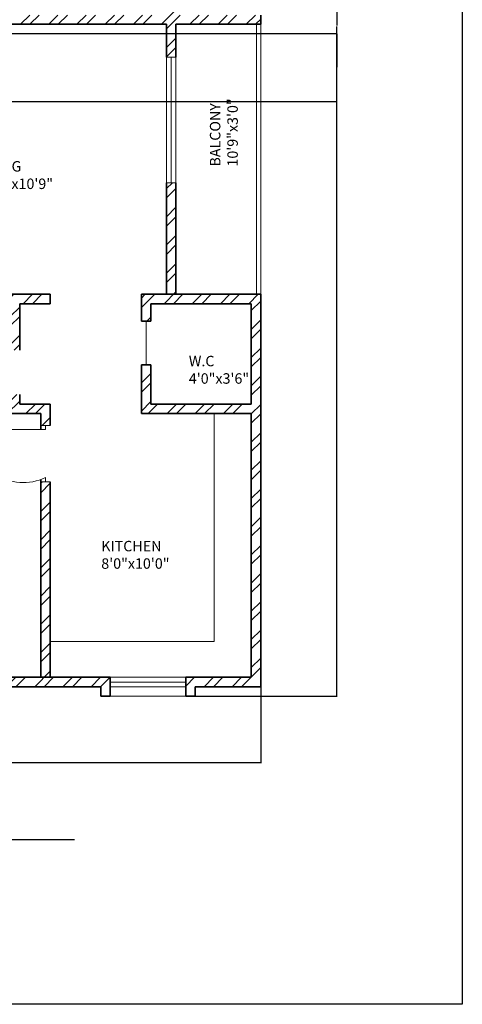
# Model space of a CAD drawing. Units: inches. Extents: x 1570 to 2186, y 1575 to 2421.
# Tile 5 of 10: x 1975 to 2186, y 1575 to 2045. Entities that reach past the tile are written whole.
import ezdxf

# ---------------------------------------------------------------- set-up
doc = ezdxf.new("R2010")
doc.units = ezdxf.units.IN
for name, color, linetype, lineweight in [('A-ANNO-DIMS', 2, 'Continuous', 18), ('A-ANNO-TTLB', 7, 'Continuous', 25), ('A-AREA-IDEN', 7, 'Continuous', 18), ('A-DOOR', 201, 'Continuous', 18), ('A-FLOR-CASE', 7, 'Continuous', 18), ('A-FLOR-HRAL', 201, 'Continuous', 18), ('A-GLAZ', 150, 'Continuous', 18), ('A-WALL', 7, 'Continuous', 35), ('A-WALL-PATT', 252, 'Continuous', 13)]:
    doc.layers.add(name, color=color, linetype=linetype, lineweight=lineweight)
doc.styles.get("Standard").update_dxf_attribs({"font": 'arial.ttf'})
doc.dimstyles.get("Standard").update_dxf_attribs({"dimtxt": 0.18, "dimasz": 0.18, "dimexe": 0.18, "dimexo": 0.0625, "dimgap": 0.09, "dimtad": 0, "dimtih": 1, "dimtoh": 1, "dimdec": 4, "dimzin": 0, "dimdsep": 46, "dimtxsty": 'Standard', "dimcen": 0.09, "dimadec": 0, "dimazin": 0, "dimtfac": 1, "dimtdec": 4, "dimtofl": 0, "dimtmove": 0, "dimatfit": 3, "dimfxl": 1, "dimtolj": 1, "dimtzin": 0, "dimarcsym": 0})

# ---------------------------------------------------------------- blocks, each defined once
blk = doc.blocks.new('WIN-60IN')
for p, q in [((0, 60), (4.5, 60)), ((0, 0), (0, 60)), ((4.5, 60), (2.25, 60)), ((2.25, 60), (2.25, 0)), ((4.5, 60), (4.5, 0)), ((2.25, 0), (0, 0)), ((0, 0), (4.5, 0))]:
    blk.add_line(p, q)
blk = doc.blocks.new('*D31')
at = {"layer": 'A-ANNO-DIMS', "color": 0, "lineweight": -2, "transparency": 16777216}
for p, q in [((1639.59, 1726.19), (1639.59, 1689.77)), ((2090.09, 1726.19), (2090.09, 1689.77)), ((1639.77, 1689.95), (1864.44, 1689.95)), ((2089.91, 1689.95), (1865.24, 1689.95))]:
    blk.add_line(p, q, dxfattribs=at)
at = {"layer": 'A-ANNO-DIMS', "color": 0, "transparency": 16777216}
for points in [[(1639.77, 1689.98), (1639.77, 1689.92), (1639.59, 1689.95)], [(2089.91, 1689.98), (2089.91, 1689.92), (2090.09, 1689.95)]]:
    blk.add_solid(points, dxfattribs=at)
at = {"layer": 'Defpoints', "color": 0, "transparency": 16777216}
for p in [(1639.59, 1726.25), (2090.09, 1726.25), (1639.59, 1689.95)]:
    blk.add_point(p, dxfattribs=at)
at = {"layer": 'A-ANNO-DIMS', "color": 0, "transparency": 16777216, "insert": (1864.84, 1689.95), "char_height": 0.18, "attachment_point": 5}
blk.add_mtext('\\A1;450.5', dxfattribs=at)
blk = doc.blocks.new('*D32')
at = {"layer": 'A-ANNO-DIMS', "color": 0, "lineweight": -2, "transparency": 16777216}
for p, q in [((2053.61, 2362.15), (2126.57, 2362.15)), ((2126.39, 2361.97), (2126.39, 2042.13)), ((2126.39, 1721.93), (2126.39, 2041.77)), ((2058.81, 1721.75), (2126.57, 1721.75))]:
    blk.add_line(p, q, dxfattribs=at)
at = {"layer": 'A-ANNO-DIMS', "color": 0, "transparency": 16777216}
for points in [[(2126.36, 2361.97), (2126.42, 2361.97), (2126.39, 2362.15)], [(2126.36, 1721.93), (2126.42, 1721.93), (2126.39, 1721.75)]]:
    blk.add_solid(points, dxfattribs=at)
at = {"layer": 'Defpoints', "color": 0, "transparency": 16777216}
for p in [(2053.54, 2362.15), (2126.39, 2362.15), (2058.75, 1721.75)]:
    blk.add_point(p, dxfattribs=at)
at = {"layer": 'A-ANNO-DIMS', "color": 0, "transparency": 16777216, "insert": (2126.39, 2041.95), "char_height": 0.18, "attachment_point": 5}
blk.add_mtext('\\A1;640.4', dxfattribs=at)
blk = doc.blocks.new('*D41')
at = {"layer": 'A-ANNO-DIMS', "color": 0, "lineweight": -2, "transparency": 16777216}
for p, q in [((1816.15, 2038.3), (2126.57, 2038.3)), ((2126.39, 2038.12), (2126.39, 2022.3)), ((2126.39, 2006.11), (2126.39, 2021.93)), ((1816.15, 2005.93), (2126.57, 2005.93))]:
    blk.add_line(p, q, dxfattribs=at)
at = {"layer": 'A-ANNO-DIMS', "color": 0, "transparency": 16777216}
for points in [[(2126.36, 2038.12), (2126.42, 2038.12), (2126.39, 2038.3)], [(2126.36, 2006.11), (2126.42, 2006.11), (2126.39, 2005.93)]]:
    blk.add_solid(points, dxfattribs=at)
at = {"layer": 'Defpoints', "color": 0, "transparency": 16777216}
for p in [(1816.09, 2038.3), (2126.39, 2038.3), (1816.09, 2005.93)]:
    blk.add_point(p, dxfattribs=at)
at = {"layer": 'A-ANNO-DIMS', "color": 0, "transparency": 16777216, "insert": (2126.39, 2022.12), "char_height": 0.18, "attachment_point": 5}
blk.add_mtext('\\A1;32.365', dxfattribs=at)

msp = doc.modelspace()

# ---------------------------------------------------------------- hatches: boundary and pattern name
at = {"layer": 'A-WALL-PATT'}
h = msp.add_hatch(dxfattribs=at)
h.set_pattern_fill('ANSI32', color=256)
h.paths.add_polyline_path([(1762.0975, 2362.1492), (1757.5975, 2362.1492), (1757.5975, 2357.6492), (1709.1163, 2357.6492), (1709.1163, 2362.1492), (1704.6163, 2362.1492), (1704.6163, 2353.1492), (1740.0886, 2353.1492), (1740.0886, 2261.8115), (1744.5886, 2261.8115), (1744.5886, 2353.1492), (1762.0975, 2353.1492)])
h.paths.add_polyline_path([(1890.2592, 2362.1492), (1885.7592, 2362.1492), (1826.5975, 2362.1492), (1822.0975, 2362.1492), (1822.0975, 2353.1492), (1862.5886, 2353.1492), (1862.5886, 2227.1492), (1744.5886, 2227.1492), (1744.5886, 2229.5389), (1742.3386, 2229.5389), (1740.0886, 2229.5389), (1740.0886, 2222.6492), (1744.5886, 2222.6492), (1756.186, 2222.6492), (1756.186, 2216.3571), (1760.686, 2216.3571), (1760.686, 2222.6492), (1832.686, 2222.6492), (1832.686, 2212.5994), (1837.186, 2212.5994), (1837.186, 2222.6492), (1893.186, 2222.6492), (1893.186, 2212.5994), (1897.686, 2212.5994), (1897.686, 2222.6492), (1989.5886, 2222.6492), (1989.5886, 2227.1492), (1989.5886, 2232.6585), (1987.3386, 2232.6585), (1985.0886, 2232.6585), (1985.0886, 2227.1492), (1867.0886, 2227.1492), (1867.0886, 2353.1492), (1890.2592, 2353.1492)])
h.paths.add_polyline_path([(1644.0886, 2353.1492), (1668.6163, 2353.1492), (1668.6163, 2362.1492), (1664.1163, 2362.1492), (1664.1163, 2358.9932), (1664.1163, 2357.6492), (1639.5886, 2357.6492), (1639.5886, 2213.8746), (1644.0886, 2213.8746), (1644.0886, 2222.6492), (1692.0886, 2222.6492), (1692.0886, 2215.9343), (1696.5886, 2215.9343), (1696.5886, 2222.6492), (1696.5886, 2227.1492), (1644.0886, 2227.1492)])
h.paths.add_polyline_path([(2013.0435, 2362.1492), (2008.5435, 2362.1492), (2008.5435, 2357.6492), (1954.7592, 2357.6492), (1954.7592, 2362.1492), (1950.2592, 2362.1492), (1950.2592, 2353.1492), (1985.0886, 2353.1492), (1985.0886, 2260.8534), (1989.5886, 2260.8534), (1989.5886, 2353.1492), (2013.0435, 2353.1492)])
h.paths.add_polyline_path([(2090.0886, 2357.6492), (2053.5435, 2357.6492), (2053.5435, 2362.1492), (2049.0435, 2362.1492), (2049.0435, 2353.1492), (2085.5886, 2353.1492), (2085.5886, 2227.1492), (2033.0886, 2227.1492), (2033.0886, 2222.6492), (2033.0886, 2214.4464), (2037.5886, 2214.4464), (2037.5886, 2222.6492), (2085.5886, 2222.6492), (2085.5886, 2212.4409), (2090.0886, 2212.4409)])
h.paths.add_polyline_path([(2090.0886, 2188.4409), (2087.8386, 2188.4409), (2085.5886, 2188.4409), (2085.5886, 2180.6492), (2037.5886, 2180.6492), (2037.5886, 2196.7956), (2033.0886, 2196.7956), (2033.0886, 2176.1492), (2037.5886, 2176.1492), (2045.0886, 2176.1492), (2045.0886, 2169.8988), (2049.5886, 2169.8988), (2049.5886, 2176.1492), (2085.5886, 2176.1492), (2085.5886, 2167.785), (2090.0886, 2167.785)])
h.paths.add_polyline_path([(2049.5886, 2147.4502), (2047.3386, 2147.4502), (2045.0886, 2147.4502), (2045.0886, 2124.4703), (2049.5886, 2124.4703)])
h.paths.add_polyline_path([(2090.0886, 2047.1492), (2049.5886, 2047.1492), (2049.5886, 2064.4703), (2045.0886, 2064.4703), (2045.0886, 2047.1492), (1918.0886, 2047.1492), (1918.0886, 2051.2061), (1913.5886, 2051.2061), (1913.5886, 2047.1492), (1913.5886, 2036.6872), (1918.0886, 2036.6872), (1918.0886, 2042.7492), (2045.0886, 2042.7492), (2045.0886, 2027.0686), (2049.5886, 2027.0686), (2049.5886, 2042.7492), (2090.0886, 2042.7492)])
h.paths.add_polyline_path([(1918.0886, 2005.9338), (1915.8386, 2005.9338), (1913.5886, 2005.9338), (1913.5886, 1913.7492), (1918.0886, 1913.7492)])
h.paths.add_polyline_path([(2090.0886, 1913.7492), (2049.5886, 1913.7492), (2045.0886, 1913.7492), (2033.0886, 1913.7492), (2033.0886, 1909.2492), (2033.0886, 1900.9803), (2037.5886, 1900.9803), (2037.5886, 1909.2492), (2085.5886, 1909.2492), (2085.5886, 1861.2492), (2037.5886, 1861.2492), (2037.5886, 1880.0859), (2033.0886, 1880.0859), (2033.0886, 1856.7492), (2085.5886, 1856.7492), (2085.5886, 1730.7492), (2054.2483, 1730.7492), (2054.2483, 1721.7492), (2058.7483, 1721.7492), (2058.7483, 1726.2492), (2090.0886, 1726.2492)])
h.paths.add_polyline_path([(2049.5886, 1967.0686), (2045.0886, 1967.0686), (2045.0886, 1913.7492), (2049.5886, 1913.7492)])
h.paths.add_polyline_path([(1989.5886, 1824.1695), (1987.3386, 1824.1695), (1985.0886, 1824.1695), (1985.0886, 1730.7492), (1989.5886, 1730.7492)])
h.paths.add_polyline_path([(1989.5886, 1861.2492), (1974.9963, 1861.2492), (1974.9963, 1865.9306), (1972.7463, 1865.9306), (1970.4963, 1865.9306), (1970.4963, 1861.2492), (1898.4963, 1861.2492), (1898.4963, 1874.2999), (1893.9963, 1874.2999), (1893.9963, 1861.2492), (1890.5886, 1861.2492), (1837.9963, 1861.2492), (1837.9963, 1874.3159), (1833.4963, 1874.3159), (1833.4963, 1861.2492), (1761.4963, 1861.2492), (1761.4963, 1865.0209), (1759.2463, 1865.0209), (1756.9963, 1865.0209), (1756.9963, 1861.2492), (1740.0886, 1861.2492), (1740.0886, 1856.7492), (1740.0886, 1850.7206), (1744.5886, 1850.7206), (1744.5886, 1856.7492), (1985.0886, 1856.7492), (1985.0886, 1851.0804), (1989.5886, 1851.0804), (1989.5886, 1856.7492)])
h.paths.add_polyline_path([(1989.5886, 1913.7492), (1740.0886, 1913.7492), (1740.0886, 1909.2492), (1756.9963, 1909.2492), (1756.9963, 1890.279), (1761.4963, 1890.279), (1761.4963, 1909.2492), (1833.4963, 1909.2492), (1833.4963, 1898.3159), (1837.9963, 1898.3159), (1837.9963, 1909.2492), (1890.5886, 1909.2492), (1893.9963, 1909.2492), (1893.9963, 1898.2999), (1898.4963, 1898.2999), (1898.4963, 1909.2492), (1970.4963, 1909.2492), (1970.4963, 1886.9887), (1974.9963, 1886.9887), (1974.9963, 1909.2492), (1989.5886, 1909.2492)])
h.paths.add_polyline_path([(1893.7344, 1730.7492), (1867.0886, 1730.7492), (1867.0886, 1856.7492), (1862.5886, 1856.7492), (1862.5886, 1730.7492), (1824.0492, 1730.7492), (1824.0492, 1721.7492), (1893.7344, 1721.7492)])
h.paths.add_polyline_path([(2018.2483, 1730.7492), (1953.7344, 1730.7492), (1953.7344, 1721.7492), (1958.2344, 1721.7492), (1958.2344, 1726.2492), (2013.7483, 1726.2492), (2013.7483, 1721.7492), (2018.2483, 1721.7492)])
h.paths.add_polyline_path([(1768.5492, 1730.7492), (1764.0492, 1730.7492), (1744.5886, 1730.7492), (1744.5886, 1819.4364), (1742.3386, 1819.4364), (1740.0886, 1819.4364), (1740.0886, 1730.7492), (1697.3801, 1730.7492), (1697.3801, 1721.7492), (1701.8801, 1721.7492), (1701.8801, 1726.2492), (1764.0492, 1726.2492), (1764.0492, 1721.7492), (1768.5492, 1721.7492)])
h.paths.add_polyline_path([(1644.0886, 1856.7492), (1639.5886, 1856.7492), (1639.5886, 1726.2492), (1657.0315, 1726.2492), (1657.0315, 1721.7492), (1661.3801, 1721.7492), (1661.3801, 1730.7492), (1644.0886, 1730.7492)])
h.paths.add_polyline_path([(1696.5886, 1876.1809), (1692.0886, 1876.1809), (1692.0886, 1861.2492), (1684.5886, 1861.2492), (1644.0886, 1861.2492), (1644.0886, 1909.2492), (1692.0886, 1909.2492), (1692.0886, 1900.3394), (1696.5886, 1900.3394), (1696.5886, 1913.7492), (1684.5886, 1913.7492), (1684.5886, 1920.2115), (1682.3386, 1920.2115), (1680.0886, 1920.2115), (1680.0886, 1913.7492), (1639.5886, 1913.7492), (1639.5886, 1856.7492), (1684.5886, 1856.7492), (1692.0886, 1856.7492), (1696.5886, 1856.7492)])
h.paths.add_polyline_path([(1684.5886, 2042.7492), (1811.5886, 2042.7492), (1811.5886, 2038.2991), (1816.0886, 2038.2991), (1816.0886, 2042.7492), (1816.0886, 2052.5708), (1813.8386, 2052.5708), (1811.5886, 2052.5708), (1811.5886, 2047.1492), (1684.5886, 2047.1492), (1684.5886, 2064.4703), (1680.0886, 2064.4703), (1680.0886, 2047.1492), (1639.5886, 2047.1492), (1639.5886, 2042.7492), (1680.0886, 2042.7492), (1680.0886, 2024.0762), (1684.5886, 2024.0762)])
h.paths.add_polyline_path([(1684.5886, 1964.0762), (1680.0886, 1964.0762), (1680.0886, 1944.6145), (1684.5886, 1944.6145)])
h.paths.add_polyline_path([(1816.0886, 1973.7492), (1876.0886, 1973.7492), (1876.0886, 1959.17), (1880.5886, 1959.17), (1880.5886, 1973.7492), (1880.5886, 1978.2492), (1816.0886, 1978.2492), (1816.0886, 2005.9338), (1813.8386, 2005.9338), (1811.5886, 2005.9338), (1811.5886, 1913.7492), (1816.0886, 1913.7492)])
h.paths.add_polyline_path([(1837.186, 2180.6492), (1837.186, 2188.5994), (1834.936, 2188.5994), (1832.686, 2188.5994), (1832.686, 2180.6492), (1760.686, 2180.6492), (1760.686, 2197.4807), (1756.186, 2197.4807), (1756.186, 2180.6492), (1744.5886, 2180.6492), (1740.0886, 2180.6492), (1740.0886, 2176.1492), (1837.186, 2176.1492)])
h.paths.add_polyline_path([(1974.186, 2196.8744), (1971.936, 2196.8744), (1969.686, 2196.8744), (1969.686, 2180.6492), (1897.686, 2180.6492), (1897.686, 2188.5994), (1895.436, 2188.5994), (1893.186, 2188.5994), (1893.186, 2180.6492), (1893.186, 2176.1492), (1974.186, 2176.1492)])
h.paths.add_polyline_path([(1918.0886, 2176.1492), (1913.5886, 2176.1492), (1913.5886, 2081.3709), (1918.0886, 2081.3709)])
h.paths.add_polyline_path([(1816.0886, 2176.1492), (1811.5886, 2176.1492), (1811.5886, 2081.3709), (1816.0886, 2081.3709)])
h.paths.add_polyline_path([(1684.5886, 2150.4939), (1682.3386, 2150.4939), (1680.0886, 2150.4939), (1680.0886, 2124.4703), (1684.5886, 2124.4703)])
h.paths.add_polyline_path([(1696.5886, 2180.6492), (1696.5886, 2197.4701), (1692.0886, 2197.4701), (1692.0886, 2180.6492), (1644.0886, 2180.6492), (1644.0886, 2189.8746), (1641.8386, 2189.8746), (1639.5886, 2189.8746), (1639.5886, 2169.814), (1644.0886, 2169.814), (1644.0886, 2176.1492), (1680.0886, 2176.1492), (1680.0886, 2171.7002), (1684.5886, 2171.7002), (1684.5886, 2176.1492), (1696.5886, 2176.1492)])

# ---------------------------------------------------------------- linework, layer by layer
at = {"layer": 'A-ANNO-TTLB'}
msp.add_line((1731.492, 1653.2104), (2001.1233, 1653.2104), dxfattribs=at)
msp.add_lwpolyline([(1569.8198, 2421.0436), (2186.3437, 2421.0436), (2186.3437, 1574.5084), (1569.8198, 1574.5084)], close=True, dxfattribs=at)
at = {"layer": 'A-DOOR'}
for p, q in [((2035.3386, 1880.0859), (2035.3386, 1900.9803)), ((1987.3386, 1849.0804), (1951.3386, 1849.0804)), ((1985.0886, 1851.0804), (1989.5886, 1851.0804)), ((1989.5886, 1851.0804), (1987.3386, 1851.0804)), ((1987.3386, 1851.0804), (1987.3386, 1849.0804)), ((1987.3386, 1824.1695), (1987.3386, 1826.1695)), ((1985.0886, 1824.1695), (1989.5886, 1824.1695)), ((1989.5886, 1824.1695), (1987.3386, 1824.1695))]:
    msp.add_line(p, q, dxfattribs=at)
msp.add_arc((1976.629, 1849.0804), 25.2904, 180, 295.053575, dxfattribs=at)
at = {"layer": 'A-FLOR-CASE'}
for p, q in [((2067.9297, 1747.7768), (2067.9297, 1856.7492)), ((1989.5886, 1747.7768), (2067.9297, 1747.7768))]:
    msp.add_line(p, q, dxfattribs=at)
at = {"layer": 'A-FLOR-HRAL'}
for p, q in [((2087.998, 1913.7492), (2087.998, 2042.7492)), ((2090.0886, 1913.7492), (2090.0886, 2042.7492))]:
    msp.add_line(p, q, dxfattribs=at)
at = {"layer": 'A-GLAZ'}
for p, q in [((2018.2483, 1730.7492), (2054.2483, 1730.7492)), ((2018.2483, 1728.4649), (2054.2483, 1728.4649)), ((2054.2483, 1726.2492), (2018.2483, 1726.2492)), ((2018.2483, 1721.7492), (2054.2483, 1721.7492))]:
    msp.add_line(p, q, dxfattribs=at)
at = {"layer": 'A-WALL'}
for p, q in [((2090.0886, 2047.1492), (2090.0886, 2042.7492)), ((2045.0886, 2042.7492), (1918.0886, 2042.7492)), ((2045.0886, 2042.7492), (2037.5886, 2042.7492)), ((2045.0886, 2042.7492), (2045.0886, 2027.0686)), ((2090.0886, 2042.7492), (2049.5886, 2042.7492)), ((2049.5886, 2042.7492), (2049.5886, 2027.0686)), ((2045.0886, 1967.0686), (2045.0886, 1913.7492)), ((2049.5886, 1967.0686), (2049.5886, 1913.7492)), ((1989.5886, 1913.7492), (1740.0886, 1913.7492)), ((1989.5886, 1909.2492), (1989.5886, 1913.7492)), ((2085.5886, 1913.7492), (2033.0886, 1913.7492)), ((2033.0886, 1909.2492), (2033.0886, 1913.7492)), ((2049.5886, 1913.7492), (2045.0886, 1913.7492)), ((2090.0886, 1913.7492), (2049.5886, 1913.7492)), ((2090.0886, 1913.7492), (2090.0886, 1726.2492)), ((1989.5886, 1909.2492), (1974.9963, 1909.2492)), ((1974.9963, 1886.9887), (1974.9963, 1909.2492)), ((2033.0886, 1900.9803), (2033.0886, 1909.2492)), ((2085.5886, 1909.2492), (2037.5886, 1909.2492)), ((2037.5886, 1909.2492), (2037.5886, 1900.9803)), ((2085.5886, 1909.2492), (2085.5886, 1861.2492)), ((2033.0886, 1900.9803), (2037.5886, 1900.9803)), ((2033.0886, 1856.7492), (2033.0886, 1880.0859)), ((2033.0886, 1880.0859), (2037.5886, 1880.0859)), ((2037.5886, 1880.0859), (2037.5886, 1861.2492)), ((1974.9963, 1861.2492), (1974.9963, 1865.9306)), ((1989.5886, 1861.2492), (1974.9963, 1861.2492)), ((1989.5886, 1856.7492), (1989.5886, 1861.2492)), ((2085.5886, 1861.2492), (2037.5886, 1861.2492)), ((1985.0886, 1856.7492), (1744.5886, 1856.7492)), ((1985.0886, 1856.7492), (1985.0886, 1849.0804)), ((1989.5886, 1856.7492), (1989.5886, 1851.0804)), ((2085.5886, 1856.7492), (2033.0886, 1856.7492)), ((2085.5886, 1856.7492), (2085.5886, 1730.7492)), ((1985.0886, 1825.2468), (1985.0886, 1730.7492)), ((1989.5886, 1824.1695), (1989.5886, 1730.7492)), ((2018.2483, 1730.7492), (1953.7344, 1730.7492)), ((2018.2483, 1730.7492), (2018.2483, 1721.7492)), ((2085.5886, 1730.7492), (2054.2483, 1730.7492)), ((2054.2483, 1721.7492), (2054.2483, 1730.7492)), ((2013.7483, 1726.2492), (1958.2344, 1726.2492)), ((2013.7483, 1721.7492), (2013.7483, 1726.2492)), ((2090.0886, 1726.2492), (2058.7483, 1726.2492)), ((2058.7483, 1721.7492), (2058.7483, 1726.2492)), ((2018.2483, 1721.7492), (2013.7483, 1721.7492)), ((2018.2483, 1721.7492), (2013.7483, 1721.7492)), ((2054.2483, 1721.7492), (2058.7483, 1721.7492)), ((2058.7483, 1721.7492), (2054.2483, 1721.7492))]:
    msp.add_line(p, q, dxfattribs=at)

# ---------------------------------------------------------------- block references
at = {"layer": 'A-GLAZ'}
msp.add_blockref('WIN-60IN', (2045.089, 1967.0684), dxfattribs=at)

# ---------------------------------------------------------------- texts
at = {"layer": 'A-AREA-IDEN', "insert": (2065.8212, 1974.7808), "char_height": 5, "attachment_point": 1, "rotation": 90}
msp.add_mtext_dynamic_manual_height_columns('BALCONY\\P10\'9"x3\'0"', width=172.761471, gutter_width=12.5, heights=[0], dxfattribs=at)
at = {"layer": 'A-AREA-IDEN', "char_height": 5, "attachment_point": 1}
for s, width, insert in [('LIVING\\P10\'7"x10\'9"', 144.692974, (1954.5434, 1977.3775)), ('W.C\\P4\'0"x3\'6"', 105.634753, (2055.7592, 1884.3493)), ('KITCHEN\\P8\'0"x10\'0"', 189.356232, (2013.9514, 1795.9363))]:
    msp.add_mtext_dynamic_manual_height_columns(s, width=width, gutter_width=12.5, heights=[0], dxfattribs=dict(at, insert=insert))

# ---------------------------------------------------------------- dimensions: what is measured, and where the dimension line sits
at = {"layer": 'A-ANNO-DIMS'}
for base, p1, p2, angle, override, picture, middle in [((2126.3886, 2362.1492), (2058.7483, 1721.7492), (2053.5435, 2362.1492), 90, {"dimdec": 1, "dimlfac": 1, "dimrnd": 0, "dimzin": 0, "dimdsep": 46, "dimlunit": 2}, '*D32', (2126.3886, 2041.9492)), ((2126.3886, 2038.2991), (1816.0886, 2005.9338), (1816.0886, 2038.2991), 90, {"dimdec": 3, "dimlfac": 1, "dimrnd": 0, "dimzin": 0, "dimdsep": 46, "dimlunit": 2}, '*D41', (2126.3886, 2022.1164)), ((1639.5886, 1689.9492), (2090.0886, 1726.2492), (1639.5886, 1726.2492), 180, {"dimdec": 1, "dimlfac": 1, "dimrnd": 0, "dimzin": 0, "dimdsep": 46, "dimlunit": 2}, '*D31', (1864.8386, 1689.9492))]:
    dim = msp.add_linear_dim(base=base, p1=p1, p2=p2, angle=angle, dimstyle='Standard', override=override, dxfattribs=at)
    dim.commit()
    dim.dimension.update_dxf_attribs({"geometry": picture, "text_midpoint": middle})

doc.saveas('drawing.dxf')
